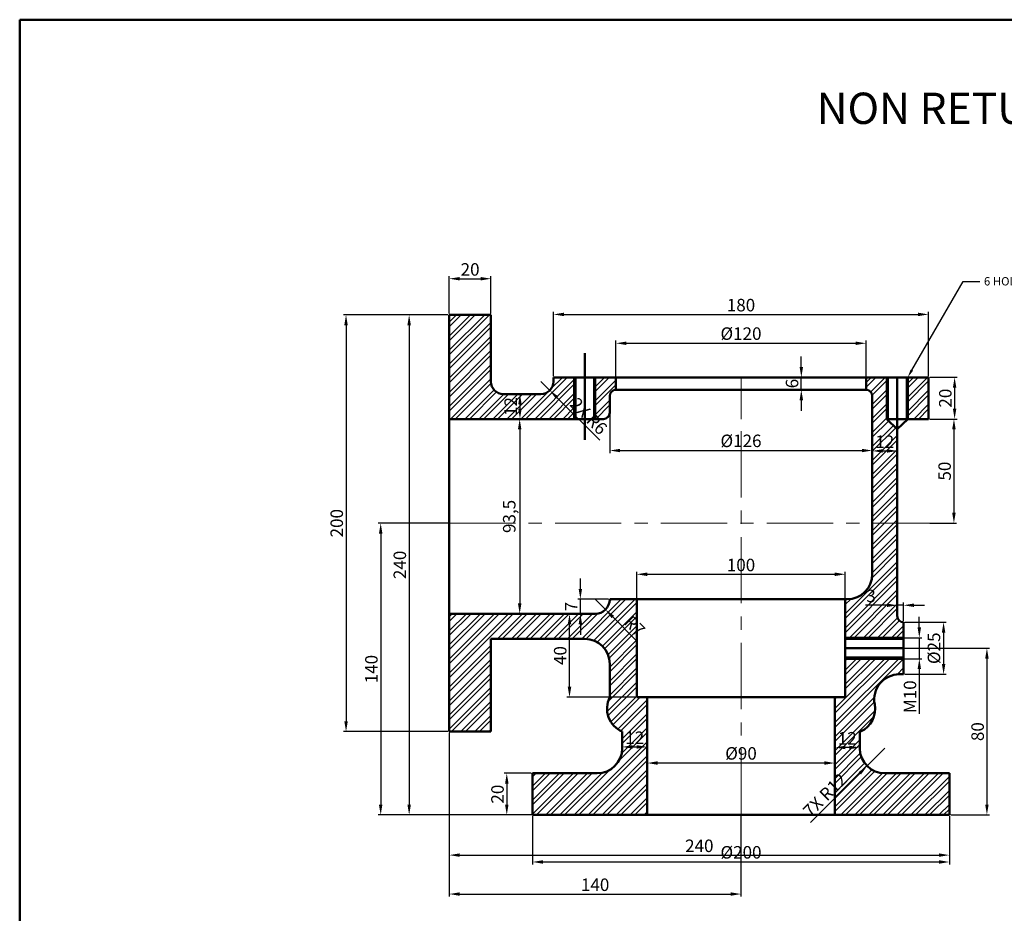
# Model space of a CAD drawing. Units: millimetres. Extents: x -907 to -46, y -312 to 510.
# Tile 2 of 3: x -907 to -434, y 81 to 510. Entities that reach past the tile are written whole.
import ezdxf
from ezdxf import colors
from ezdxf.entities.mleader import LeaderData, LeaderLine
from ezdxf.math import Vec2, Vec3

# ---------------------------------------------------------------- set-up
doc = ezdxf.new("R2010")
doc.units = ezdxf.units.MM
doc.linetypes.add('CENTER', pattern=[50.8, 31.75, -6.35, 6.35, -6.35])
for name, color, linetype, lineweight in [('M-CNTR', 1, 'CENTER', 18), ('M-DIMS', 2, 'Continuous', 25), ('M-HATC', 8, 'Continuous', 18), ('M-OUTL', 7, 'Continuous', 50), ('M-TEXT', 3, 'Continuous', 25), ('M-TTLB', 7, 'Continuous', 50)]:
    doc.layers.add(name, color=color, linetype=linetype, lineweight=lineweight)
doc.styles.get("Standard").update_dxf_attribs({"font": 'arial.ttf'})
doc.dimstyles.new('ISO-25', dxfattribs={"dimtxt": 6, "dimasz": 5, "dimexe": 1.25, "dimexo": 0.625, "dimtad": 1, "dimtxsty": 'Standard', "dimcen": 2.5, "dimadec": 0, "dimazin": 0, "dimtfac": 1, "dimtmove": 0, "dimatfit": 3, "dimfxl": 1, "dimarcsym": 0})

# ---------------------------------------------------------------- blocks, each defined once
blk = doc.blocks.new('*D1')
at = {"layer": 'Defpoints', "color": 0, "transparency": 16777216}
for p in [(-660.8, 128.33), (-460.8, 128.33), (-460.8, 105.78)]:
    blk.add_point(p, dxfattribs=at)
at = {"layer": 'M-DIMS', "color": 0, "lineweight": -2, "transparency": 16777216}
for p, q in [((-660.8, 127.7), (-660.8, 104.53)), ((-460.8, 127.7), (-460.8, 104.53)), ((-655.8, 105.78), (-465.8, 105.78))]:
    blk.add_line(p, q, dxfattribs=at)
at = {"layer": 'M-DIMS', "color": 0, "transparency": 16777216}
for points in [[(-655.8, 106.62), (-655.8, 104.95), (-660.8, 105.78)], [(-465.8, 106.62), (-465.8, 104.95), (-460.8, 105.78)]]:
    blk.add_solid(points, dxfattribs=at)
at = {"layer": 'M-DIMS', "color": 0, "transparency": 16777216, "insert": (-560.8, 109.64), "char_height": 6, "attachment_point": 5}
blk.add_mtext('%%C200', dxfattribs=at)
blk = doc.blocks.new('*D2')
at = {"layer": 'Defpoints', "color": 0, "transparency": 16777216}
for p in [(-700.8, 168.33), (-560.8, 128.33), (-560.8, 90.4)]:
    blk.add_point(p, dxfattribs=at)
at = {"layer": 'M-DIMS', "color": 0, "lineweight": -2, "transparency": 16777216}
for p, q in [((-700.8, 167.7), (-700.8, 89.15)), ((-560.8, 127.7), (-560.8, 89.15)), ((-695.8, 90.4), (-565.8, 90.4))]:
    blk.add_line(p, q, dxfattribs=at)
at = {"layer": 'M-DIMS', "color": 0, "transparency": 16777216}
for points in [[(-695.8, 91.23), (-695.8, 89.56), (-700.8, 90.4)], [(-565.8, 91.23), (-565.8, 89.56), (-560.8, 90.4)]]:
    blk.add_solid(points, dxfattribs=at)
at = {"layer": 'M-DIMS', "color": 0, "transparency": 16777216, "insert": (-630.8, 94.08), "char_height": 6, "attachment_point": 5}
blk.add_mtext('140', dxfattribs=at)
blk = doc.blocks.new('*D3')
at = {"layer": 'Defpoints', "color": 0, "transparency": 16777216}
for p in [(-605.8, 156.58), (-515.8, 156.58), (-605.8, 153.25)]:
    blk.add_point(p, dxfattribs=at)
at = {"layer": 'M-DIMS', "color": 0, "lineweight": -2, "transparency": 16777216}
for p, q in [((-605.8, 155.95), (-605.8, 152)), ((-515.8, 155.95), (-515.8, 152)), ((-520.8, 153.25), (-600.8, 153.25))]:
    blk.add_line(p, q, dxfattribs=at)
at = {"layer": 'M-DIMS', "color": 0, "transparency": 16777216}
for points in [[(-600.8, 154.09), (-600.8, 152.42), (-605.8, 153.25)], [(-520.8, 154.09), (-520.8, 152.42), (-515.8, 153.25)]]:
    blk.add_solid(points, dxfattribs=at)
at = {"layer": 'M-DIMS', "color": 0, "transparency": 16777216, "insert": (-560.8, 157.11), "char_height": 6, "attachment_point": 5}
blk.add_mtext('%%C90', dxfattribs=at)
blk = doc.blocks.new('*D4')
at = {"layer": 'Defpoints', "color": 0, "transparency": 16777216}
for p in [(-605.8, 160.99), (-617.8, 160.33), (-605.8, 160.33)]:
    blk.add_point(p, dxfattribs=at)
at = {"layer": 'M-DIMS', "color": 0, "lineweight": -2, "transparency": 16777216}
for p, q in [((-617.8, 160.95), (-617.8, 162.24)), ((-612.8, 160.99), (-610.8, 160.99)), ((-605.8, 160.95), (-605.8, 162.24))]:
    blk.add_line(p, q, dxfattribs=at)
at = {"layer": 'M-DIMS', "color": 0, "transparency": 16777216}
for points in [[(-612.8, 161.83), (-612.8, 160.16), (-617.8, 160.99)], [(-610.8, 161.83), (-610.8, 160.16), (-605.8, 160.99)]]:
    blk.add_solid(points, dxfattribs=at)
at = {"layer": 'M-DIMS', "color": 0, "transparency": 16777216, "insert": (-611.8, 164.63), "char_height": 6, "attachment_point": 5}
blk.add_mtext('12', dxfattribs=at)
blk = doc.blocks.new('*D5')
at = {"layer": 'Defpoints', "color": 0, "transparency": 16777216}
for p in [(-643.1, 224.83), (-630.8, 224.83), (-610.8, 184.83)]:
    blk.add_point(p, dxfattribs=at)
at = {"layer": 'M-DIMS', "color": 0, "lineweight": -2, "transparency": 16777216}
for p, q in [((-631.42, 224.83), (-644.35, 224.83)), ((-643.1, 189.83), (-643.1, 219.83)), ((-611.42, 184.83), (-644.35, 184.83))]:
    blk.add_line(p, q, dxfattribs=at)
at = {"layer": 'M-DIMS', "color": 0, "transparency": 16777216}
for points in [[(-643.93, 219.83), (-642.26, 219.83), (-643.1, 224.83)], [(-643.93, 189.83), (-642.26, 189.83), (-643.1, 184.83)]]:
    blk.add_solid(points, dxfattribs=at)
at = {"layer": 'M-DIMS', "color": 0, "transparency": 16777216, "insert": (-646.79, 204.83), "char_height": 6, "attachment_point": 5, "rotation": 90}
blk.add_mtext('40', dxfattribs=at)
blk = doc.blocks.new('*D6')
at = {"layer": 'Defpoints', "color": 0, "transparency": 16777216}
for p in [(-482.8, 208.33), (-460.8, 128.33), (-442.79, 128.33)]:
    blk.add_point(p, dxfattribs=at)
at = {"layer": 'M-DIMS', "color": 0, "lineweight": -2, "transparency": 16777216}
for p, q in [((-482.17, 208.33), (-441.54, 208.33)), ((-442.79, 203.33), (-442.79, 133.33)), ((-460.17, 128.33), (-441.54, 128.33))]:
    blk.add_line(p, q, dxfattribs=at)
at = {"layer": 'M-DIMS', "color": 0, "transparency": 16777216}
for points in [[(-443.62, 203.33), (-441.96, 203.33), (-442.79, 208.33)], [(-443.62, 133.33), (-441.96, 133.33), (-442.79, 128.33)]]:
    blk.add_solid(points, dxfattribs=at)
at = {"layer": 'M-DIMS', "color": 0, "transparency": 16777216, "insert": (-446.48, 168.33), "char_height": 6, "attachment_point": 5, "rotation": 90}
blk.add_mtext('80', dxfattribs=at)
blk = doc.blocks.new('*D7')
at = {"layer": 'Defpoints', "color": 0, "transparency": 16777216}
for p in [(-515.8, 164.33), (-515.8, 160.72), (-503.8, 164.33)]:
    blk.add_point(p, dxfattribs=at)
at = {"layer": 'M-DIMS', "color": 0, "lineweight": -2, "transparency": 16777216}
for p, q in [((-515.8, 163.7), (-515.8, 159.47)), ((-508.8, 160.72), (-510.8, 160.72)), ((-503.8, 163.7), (-503.8, 159.47))]:
    blk.add_line(p, q, dxfattribs=at)
at = {"layer": 'M-DIMS', "color": 0, "transparency": 16777216}
for points in [[(-510.8, 161.55), (-510.8, 159.89), (-515.8, 160.72)], [(-508.8, 161.55), (-508.8, 159.89), (-503.8, 160.72)]]:
    blk.add_solid(points, dxfattribs=at)
at = {"layer": 'M-DIMS', "color": 0, "transparency": 16777216, "insert": (-509.8, 164.36), "char_height": 6, "attachment_point": 5}
blk.add_mtext('12', dxfattribs=at)
blk = doc.blocks.new('*D8')
at = {"layer": 'Defpoints', "color": 0, "transparency": 16777216}
for p in [(-482.8, 213.33), (-482.8, 203.33), (-475.23, 203.33)]:
    blk.add_point(p, dxfattribs=at)
at = {"layer": 'M-DIMS', "color": 0, "lineweight": -2, "transparency": 16777216}
for p, q in [((-475.23, 218.33), (-475.23, 223.33)), ((-482.17, 213.33), (-473.98, 213.33)), ((-475.23, 213.33), (-475.23, 203.33)), ((-482.17, 203.33), (-473.98, 203.33)), ((-475.23, 198.33), (-475.23, 176.79))]:
    blk.add_line(p, q, dxfattribs=at)
at = {"layer": 'M-DIMS', "color": 0, "transparency": 16777216}
for points in [[(-476.06, 218.33), (-474.4, 218.33), (-475.23, 213.33)], [(-476.06, 198.33), (-474.4, 198.33), (-475.23, 203.33)]]:
    blk.add_solid(points, dxfattribs=at)
at = {"layer": 'M-DIMS', "color": 0, "transparency": 16777216, "insert": (-478.92, 185.06), "char_height": 6, "attachment_point": 5, "rotation": 90}
blk.add_mtext('M10', dxfattribs=at)
blk = doc.blocks.new('*D9')
at = {"layer": 'Defpoints', "color": 0, "transparency": 16777216}
for p in [(-482.8, 220.83), (-482.8, 195.83), (-463.58, 195.83)]:
    blk.add_point(p, dxfattribs=at)
at = {"layer": 'M-DIMS', "color": 0, "lineweight": -2, "transparency": 16777216}
for p, q in [((-482.17, 220.83), (-462.33, 220.83)), ((-463.58, 215.83), (-463.58, 200.83)), ((-482.17, 195.83), (-462.33, 195.83))]:
    blk.add_line(p, q, dxfattribs=at)
at = {"layer": 'M-DIMS', "color": 0, "transparency": 16777216}
for points in [[(-464.41, 215.83), (-462.74, 215.83), (-463.58, 220.83)], [(-464.41, 200.83), (-462.74, 200.83), (-463.58, 195.83)]]:
    blk.add_solid(points, dxfattribs=at)
at = {"layer": 'M-DIMS', "color": 0, "transparency": 16777216, "insert": (-467.43, 208.33), "char_height": 6, "attachment_point": 5, "rotation": 90}
blk.add_mtext('%%C25', dxfattribs=at)
blk = doc.blocks.new('*D10')
at = {"layer": 'Defpoints', "color": 0, "transparency": 16777216}
for p in [(-510.8, 243.83), (-610.8, 231.83), (-510.8, 231.83)]:
    blk.add_point(p, dxfattribs=at)
at = {"layer": 'M-DIMS', "color": 0, "lineweight": -2, "transparency": 16777216}
for p, q in [((-610.8, 232.45), (-610.8, 245.08)), ((-605.8, 243.83), (-515.8, 243.83)), ((-510.8, 232.45), (-510.8, 245.08))]:
    blk.add_line(p, q, dxfattribs=at)
at = {"layer": 'M-DIMS', "color": 0, "transparency": 16777216}
for points in [[(-605.8, 244.66), (-605.8, 242.99), (-610.8, 243.83)], [(-515.8, 244.66), (-515.8, 242.99), (-510.8, 243.83)]]:
    blk.add_solid(points, dxfattribs=at)
at = {"layer": 'M-DIMS', "color": 0, "transparency": 16777216, "insert": (-560.8, 247.51), "char_height": 6, "attachment_point": 5}
blk.add_mtext('100', dxfattribs=at)
blk = doc.blocks.new('*D11')
at = {"layer": 'Defpoints', "color": 0, "transparency": 16777216}
for p in [(-637.89, 231.83), (-623.8, 231.83), (-630.8, 224.83)]:
    blk.add_point(p, dxfattribs=at)
at = {"layer": 'M-DIMS', "color": 0, "lineweight": -2, "transparency": 16777216}
for p, q in [((-637.89, 236.83), (-637.89, 241.83)), ((-624.42, 231.83), (-639.14, 231.83)), ((-637.89, 224.83), (-637.89, 231.83)), ((-631.42, 224.83), (-639.14, 224.83)), ((-637.89, 219.83), (-637.89, 214.83))]:
    blk.add_line(p, q, dxfattribs=at)
at = {"layer": 'M-DIMS', "color": 0, "transparency": 16777216}
for points in [[(-638.72, 236.83), (-637.05, 236.83), (-637.89, 231.83)], [(-638.72, 219.83), (-637.05, 219.83), (-637.89, 224.83)]]:
    blk.add_solid(points, dxfattribs=at)
at = {"layer": 'M-DIMS', "color": 0, "transparency": 16777216, "insert": (-641.51, 228.33), "char_height": 6, "attachment_point": 5, "rotation": 90}
blk.add_mtext('7', dxfattribs=at)
blk = doc.blocks.new('*D12')
at = {"layer": 'Defpoints', "color": 0, "transparency": 16777216}
for p in [(-700.8, 268.33), (-733.7, 128.33), (-660.8, 128.33)]:
    blk.add_point(p, dxfattribs=at)
at = {"layer": 'M-DIMS', "color": 0, "lineweight": -2, "transparency": 16777216}
for p, q in [((-701.42, 268.33), (-734.95, 268.33)), ((-733.7, 263.33), (-733.7, 133.33)), ((-661.42, 128.33), (-734.95, 128.33))]:
    blk.add_line(p, q, dxfattribs=at)
at = {"layer": 'M-DIMS', "color": 0, "transparency": 16777216}
for points in [[(-734.54, 263.33), (-732.87, 263.33), (-733.7, 268.33)], [(-734.54, 133.33), (-732.87, 133.33), (-733.7, 128.33)]]:
    blk.add_solid(points, dxfattribs=at)
at = {"layer": 'M-DIMS', "color": 0, "transparency": 16777216, "insert": (-737.39, 198.33), "char_height": 6, "attachment_point": 5, "rotation": 90}
blk.add_mtext('140', dxfattribs=at)
blk = doc.blocks.new('*D13')
at = {"layer": 'Defpoints', "color": 0, "transparency": 16777216}
for p in [(-700.8, 368.33), (-750.33, 168.33), (-700.8, 168.33)]:
    blk.add_point(p, dxfattribs=at)
at = {"layer": 'M-DIMS', "color": 0, "lineweight": -2, "transparency": 16777216}
for p, q in [((-701.42, 368.33), (-751.58, 368.33)), ((-750.33, 363.33), (-750.33, 173.33)), ((-701.42, 168.33), (-751.58, 168.33))]:
    blk.add_line(p, q, dxfattribs=at)
at = {"layer": 'M-DIMS', "color": 0, "transparency": 16777216}
for points in [[(-751.16, 363.33), (-749.5, 363.33), (-750.33, 368.33)], [(-751.16, 173.33), (-749.5, 173.33), (-750.33, 168.33)]]:
    blk.add_solid(points, dxfattribs=at)
at = {"layer": 'M-DIMS', "color": 0, "transparency": 16777216, "insert": (-754.02, 268.33), "char_height": 6, "attachment_point": 5, "rotation": 90}
blk.add_mtext('200', dxfattribs=at)
blk = doc.blocks.new('*D14')
at = {"layer": 'Defpoints', "color": 0, "transparency": 16777216}
for p in [(-665.8, 330.33), (-666.88, 318.33), (-665.8, 318.33)]:
    blk.add_point(p, dxfattribs=at)
at = {"layer": 'M-DIMS', "color": 0, "lineweight": -2, "transparency": 16777216}
for p, q in [((-666.42, 330.33), (-668.13, 330.33)), ((-666.88, 325.33), (-666.88, 323.33)), ((-666.42, 318.33), (-668.13, 318.33))]:
    blk.add_line(p, q, dxfattribs=at)
at = {"layer": 'M-DIMS', "color": 0, "transparency": 16777216}
for points in [[(-667.72, 325.33), (-666.05, 325.33), (-666.88, 330.33)], [(-667.72, 323.33), (-666.05, 323.33), (-666.88, 318.33)]]:
    blk.add_solid(points, dxfattribs=at)
at = {"layer": 'M-DIMS', "color": 0, "transparency": 16777216, "insert": (-670.52, 324.33), "char_height": 6, "attachment_point": 5, "rotation": 90}
blk.add_mtext('12', dxfattribs=at)
blk = doc.blocks.new('*D15')
at = {"layer": 'Defpoints', "color": 0, "transparency": 16777216}
for p in [(-680.8, 385.65), (-700.8, 368.33), (-680.8, 368.33)]:
    blk.add_point(p, dxfattribs=at)
at = {"layer": 'M-DIMS', "color": 0, "lineweight": -2, "transparency": 16777216}
for p, q in [((-700.8, 368.95), (-700.8, 386.9)), ((-695.8, 385.65), (-685.8, 385.65)), ((-680.8, 368.95), (-680.8, 386.9))]:
    blk.add_line(p, q, dxfattribs=at)
at = {"layer": 'M-DIMS', "color": 0, "transparency": 16777216}
for points in [[(-695.8, 386.48), (-695.8, 384.81), (-700.8, 385.65)], [(-685.8, 386.48), (-685.8, 384.81), (-680.8, 385.65)]]:
    blk.add_solid(points, dxfattribs=at)
at = {"layer": 'M-DIMS', "color": 0, "transparency": 16777216, "insert": (-690.8, 389.33), "char_height": 6, "attachment_point": 5}
blk.add_mtext('20', dxfattribs=at)
blk = doc.blocks.new('*D16')
at = {"layer": 'Defpoints', "color": 0, "transparency": 16777216}
for p in [(-470.8, 368.52), (-650.8, 338.33), (-470.8, 338.33)]:
    blk.add_point(p, dxfattribs=at)
at = {"layer": 'M-DIMS', "color": 0, "lineweight": -2, "transparency": 16777216}
for p, q in [((-650.8, 338.95), (-650.8, 369.77)), ((-470.8, 338.95), (-470.8, 369.77)), ((-645.8, 368.52), (-475.8, 368.52))]:
    blk.add_line(p, q, dxfattribs=at)
at = {"layer": 'M-DIMS', "color": 0, "transparency": 16777216}
for points in [[(-645.8, 369.35), (-645.8, 367.68), (-650.8, 368.52)], [(-475.8, 369.35), (-475.8, 367.68), (-470.8, 368.52)]]:
    blk.add_solid(points, dxfattribs=at)
at = {"layer": 'M-DIMS', "color": 0, "transparency": 16777216, "insert": (-560.8, 372.2), "char_height": 6, "attachment_point": 5}
blk.add_mtext('180', dxfattribs=at)
blk = doc.blocks.new('*D17')
at = {"layer": 'Defpoints', "color": 0, "transparency": 16777216}
for p in [(-623.8, 321.33), (-497.8, 321.33), (-497.8, 303.21)]:
    blk.add_point(p, dxfattribs=at)
at = {"layer": 'M-DIMS', "color": 0, "lineweight": -2, "transparency": 16777216}
for p, q in [((-623.8, 320.7), (-623.8, 301.96)), ((-497.8, 320.7), (-497.8, 301.96)), ((-618.8, 303.21), (-502.8, 303.21))]:
    blk.add_line(p, q, dxfattribs=at)
at = {"layer": 'M-DIMS', "color": 0, "transparency": 16777216}
for points in [[(-618.8, 304.04), (-618.8, 302.38), (-623.8, 303.21)], [(-502.8, 304.04), (-502.8, 302.38), (-497.8, 303.21)]]:
    blk.add_solid(points, dxfattribs=at)
at = {"layer": 'M-DIMS', "color": 0, "transparency": 16777216, "insert": (-560.8, 307.07), "char_height": 6, "attachment_point": 5}
blk.add_mtext('%%C126', dxfattribs=at)
blk = doc.blocks.new('*D18')
at = {"layer": 'Defpoints', "color": 0, "transparency": 16777216}
for p in [(-470.8, 338.33), (-470.8, 318.33), (-458.29, 318.33)]:
    blk.add_point(p, dxfattribs=at)
at = {"layer": 'M-DIMS', "color": 0, "lineweight": -2, "transparency": 16777216}
for p, q in [((-470.17, 338.33), (-457.04, 338.33)), ((-458.29, 333.33), (-458.29, 323.33)), ((-470.17, 318.33), (-457.04, 318.33))]:
    blk.add_line(p, q, dxfattribs=at)
at = {"layer": 'M-DIMS', "color": 0, "transparency": 16777216}
for points in [[(-459.12, 333.33), (-457.46, 333.33), (-458.29, 338.33)], [(-459.12, 323.33), (-457.46, 323.33), (-458.29, 318.33)]]:
    blk.add_solid(points, dxfattribs=at)
at = {"layer": 'M-DIMS', "color": 0, "transparency": 16777216, "insert": (-461.98, 328.33), "char_height": 6, "attachment_point": 5, "rotation": 90}
blk.add_mtext('20', dxfattribs=at)
blk = doc.blocks.new('*D19')
at = {"layer": 'Defpoints', "color": 0, "transparency": 16777216}
for p in [(-500.8, 354.67), (-620.8, 332.33), (-500.8, 332.33)]:
    blk.add_point(p, dxfattribs=at)
at = {"layer": 'M-DIMS', "color": 0, "lineweight": -2, "transparency": 16777216}
for p, q in [((-620.8, 332.95), (-620.8, 355.92)), ((-615.8, 354.67), (-505.8, 354.67)), ((-500.8, 332.95), (-500.8, 355.92))]:
    blk.add_line(p, q, dxfattribs=at)
at = {"layer": 'M-DIMS', "color": 0, "transparency": 16777216}
for points in [[(-615.8, 355.5), (-615.8, 353.84), (-620.8, 354.67)], [(-505.8, 355.5), (-505.8, 353.84), (-500.8, 354.67)]]:
    blk.add_solid(points, dxfattribs=at)
at = {"layer": 'M-DIMS', "color": 0, "transparency": 16777216, "insert": (-560.8, 358.53), "char_height": 6, "attachment_point": 5}
blk.add_mtext('%%C120', dxfattribs=at)
blk = doc.blocks.new('*D20')
at = {"layer": 'Defpoints', "color": 0, "transparency": 16777216}
for p in [(-539.22, 338.33), (-531.85, 338.33), (-539.22, 332.33)]:
    blk.add_point(p, dxfattribs=at)
at = {"layer": 'M-DIMS', "color": 0, "lineweight": -2, "transparency": 16777216}
for p, q in [((-531.85, 343.33), (-531.85, 348.33)), ((-538.6, 338.33), (-530.6, 338.33)), ((-531.85, 332.33), (-531.85, 338.33)), ((-538.6, 332.33), (-530.6, 332.33)), ((-531.85, 327.33), (-531.85, 322.33))]:
    blk.add_line(p, q, dxfattribs=at)
at = {"layer": 'M-DIMS', "color": 0, "transparency": 16777216}
for points in [[(-532.68, 343.33), (-531.01, 343.33), (-531.85, 338.33)], [(-532.68, 327.33), (-531.01, 327.33), (-531.85, 332.33)]]:
    blk.add_solid(points, dxfattribs=at)
at = {"layer": 'M-DIMS', "color": 0, "transparency": 16777216, "insert": (-535.53, 335.33), "char_height": 6, "attachment_point": 5, "rotation": 90}
blk.add_mtext('6', dxfattribs=at)
blk = doc.blocks.new('*D21')
at = {"layer": 'Defpoints', "color": 0, "transparency": 16777216}
for p in [(-497.8, 306.37), (-485.8, 306.37), (-485.8, 303)]:
    blk.add_point(p, dxfattribs=at)
at = {"layer": 'M-DIMS', "color": 0, "lineweight": -2, "transparency": 16777216}
for p, q in [((-497.8, 305.74), (-497.8, 301.75)), ((-492.8, 303), (-490.8, 303)), ((-485.8, 305.74), (-485.8, 301.75))]:
    blk.add_line(p, q, dxfattribs=at)
at = {"layer": 'M-DIMS', "color": 0, "transparency": 16777216}
for points in [[(-492.8, 303.84), (-492.8, 302.17), (-497.8, 303)], [(-490.8, 303.84), (-490.8, 302.17), (-485.8, 303)]]:
    blk.add_solid(points, dxfattribs=at)
at = {"layer": 'M-DIMS', "color": 0, "transparency": 16777216, "insert": (-491.8, 306.64), "char_height": 6, "attachment_point": 5}
blk.add_mtext('12', dxfattribs=at)
blk = doc.blocks.new('*D22')
at = {"layer": 'Defpoints', "color": 0, "transparency": 16777216}
for p in [(-485.8, 228.96), (-485.8, 223.83), (-482.8, 220.83)]:
    blk.add_point(p, dxfattribs=at)
at = {"layer": 'M-DIMS', "color": 0, "lineweight": -2, "transparency": 16777216}
for p, q in [((-490.8, 228.96), (-500.98, 228.96)), ((-485.8, 224.45), (-485.8, 230.21)), ((-482.8, 228.96), (-485.8, 228.96)), ((-482.8, 221.45), (-482.8, 230.21)), ((-477.8, 228.96), (-472.8, 228.96))]:
    blk.add_line(p, q, dxfattribs=at)
at = {"layer": 'M-DIMS', "color": 0, "transparency": 16777216}
for points in [[(-490.8, 229.79), (-490.8, 228.12), (-485.8, 228.96)], [(-477.8, 229.79), (-477.8, 228.12), (-482.8, 228.96)]]:
    blk.add_solid(points, dxfattribs=at)
at = {"layer": 'M-DIMS', "color": 0, "transparency": 16777216, "insert": (-498.39, 232.65), "char_height": 6, "attachment_point": 5}
blk.add_mtext('3', dxfattribs=at)
blk = doc.blocks.new('*D23')
at = {"layer": 'Defpoints', "color": 0, "transparency": 16777216}
for p in [(-675.8, 318.33), (-675.8, 224.83), (-667, 224.83)]:
    blk.add_point(p, dxfattribs=at)
at = {"layer": 'M-DIMS', "color": 0, "lineweight": -2, "transparency": 16777216}
for p, q in [((-675.17, 318.33), (-665.75, 318.33)), ((-667, 313.33), (-667, 229.83)), ((-675.17, 224.83), (-665.75, 224.83))]:
    blk.add_line(p, q, dxfattribs=at)
at = {"layer": 'M-DIMS', "color": 0, "transparency": 16777216}
for points in [[(-667.84, 313.33), (-666.17, 313.33), (-667, 318.33)], [(-667.84, 229.83), (-666.17, 229.83), (-667, 224.83)]]:
    blk.add_solid(points, dxfattribs=at)
at = {"layer": 'M-DIMS', "color": 0, "transparency": 16777216, "insert": (-671.23, 271.58), "char_height": 6, "attachment_point": 5, "rotation": 90}
blk.add_mtext('93,5', dxfattribs=at)
blk = doc.blocks.new('*D44')
at = {"layer": 'Defpoints', "color": 0, "transparency": 16777216}
for p in [(-660.8, 148.33), (-673.19, 128.33), (-660.8, 128.33)]:
    blk.add_point(p, dxfattribs=at)
at = {"layer": 'M-DIMS', "color": 0, "lineweight": -2, "transparency": 16777216}
for p, q in [((-661.42, 148.33), (-674.44, 148.33)), ((-673.19, 143.33), (-673.19, 133.33)), ((-661.42, 128.33), (-674.44, 128.33))]:
    blk.add_line(p, q, dxfattribs=at)
at = {"layer": 'M-DIMS', "color": 0, "transparency": 16777216}
for points in [[(-674.02, 143.33), (-672.35, 143.33), (-673.19, 148.33)], [(-674.02, 133.33), (-672.35, 133.33), (-673.19, 128.33)]]:
    blk.add_solid(points, dxfattribs=at)
at = {"layer": 'M-DIMS', "color": 0, "transparency": 16777216, "insert": (-676.87, 138.33), "char_height": 6, "attachment_point": 5, "rotation": 90}
blk.add_mtext('20', dxfattribs=at)
blk = doc.blocks.new('*D45')
at = {"layer": 'Defpoints', "color": 0, "transparency": 16777216}
for p in [(-470.8, 318.33), (-470.8, 268.33), (-458.62, 268.33)]:
    blk.add_point(p, dxfattribs=at)
at = {"layer": 'M-DIMS', "color": 0, "lineweight": -2, "transparency": 16777216}
for p, q in [((-470.17, 318.33), (-457.37, 318.33)), ((-458.62, 313.33), (-458.62, 273.33)), ((-470.17, 268.33), (-457.37, 268.33))]:
    blk.add_line(p, q, dxfattribs=at)
at = {"layer": 'M-DIMS', "color": 0, "transparency": 16777216}
for points in [[(-459.46, 313.33), (-457.79, 313.33), (-458.62, 318.33)], [(-459.46, 273.33), (-457.79, 273.33), (-458.62, 268.33)]]:
    blk.add_solid(points, dxfattribs=at)
at = {"layer": 'M-DIMS', "color": 0, "transparency": 16777216, "insert": (-462.31, 293.33), "char_height": 6, "attachment_point": 5, "rotation": 90}
blk.add_mtext('50', dxfattribs=at)
blk = doc.blocks.new('*D55')
at = {"layer": 'Defpoints', "color": 0, "transparency": 16777216}
for p in [(-700.8, 368.33), (-720.05, 128.33), (-460.8, 128.33)]:
    blk.add_point(p, dxfattribs=at)
at = {"layer": 'M-DIMS', "color": 0, "lineweight": -2, "transparency": 16777216}
for p, q in [((-701.42, 368.33), (-721.3, 368.33)), ((-720.05, 363.33), (-720.05, 133.33)), ((-461.42, 128.33), (-721.3, 128.33))]:
    blk.add_line(p, q, dxfattribs=at)
at = {"layer": 'M-DIMS', "color": 0, "transparency": 16777216}
for points in [[(-720.88, 363.33), (-719.21, 363.33), (-720.05, 368.33)], [(-720.88, 133.33), (-719.21, 133.33), (-720.05, 128.33)]]:
    blk.add_solid(points, dxfattribs=at)
at = {"layer": 'M-DIMS', "color": 0, "transparency": 16777216, "insert": (-723.74, 248.33), "char_height": 6, "attachment_point": 5, "rotation": 90}
blk.add_mtext('240', dxfattribs=at)
blk = doc.blocks.new('*D56')
at = {"layer": 'Defpoints', "color": 0, "transparency": 16777216}
for p in [(-700.8, 168.33), (-460.8, 128.33), (-460.8, 109.08)]:
    blk.add_point(p, dxfattribs=at)
at = {"layer": 'M-DIMS', "color": 0, "lineweight": -2, "transparency": 16777216}
for p, q in [((-700.8, 167.7), (-700.8, 107.83)), ((-460.8, 127.7), (-460.8, 107.83)), ((-695.8, 109.08), (-465.8, 109.08))]:
    blk.add_line(p, q, dxfattribs=at)
at = {"layer": 'M-DIMS', "color": 0, "transparency": 16777216}
for points in [[(-695.8, 109.91), (-695.8, 108.24), (-700.8, 109.08)], [(-465.8, 109.91), (-465.8, 108.24), (-460.8, 109.08)]]:
    blk.add_solid(points, dxfattribs=at)
at = {"layer": 'M-DIMS', "color": 0, "transparency": 16777216, "insert": (-580.8, 112.76), "char_height": 6, "attachment_point": 5}
blk.add_mtext('240', dxfattribs=at)
blk = doc.blocks.new('*D61')
at = {"layer": 'Defpoints', "color": 0, "transparency": 16777216}
for p in [(-491.8, 160.33), (-500.28, 151.84)]:
    blk.add_point(p, dxfattribs=at)
at = {"layer": 'M-DIMS', "color": 0, "lineweight": -2, "transparency": 16777216}
for p, q in [((-491.8, 160.33), (-500.28, 151.84)), ((-527.41, 124.71), (-503.82, 148.3))]:
    blk.add_line(p, q, dxfattribs=at)
at = {"layer": 'M-DIMS', "color": 0, "transparency": 16777216}
blk.add_solid([(-504.41, 148.89), (-503.23, 147.72), (-500.28, 151.84)], dxfattribs=at)
at = {"layer": 'M-DIMS', "color": 0, "transparency": 16777216, "insert": (-519.96, 137.31), "char_height": 6, "attachment_point": 5, "rotation": 44.9999}
blk.add_mtext('7X R12', dxfattribs=at)
blk = doc.blocks.new('*D62')
at = {"layer": 'Defpoints', "color": 0, "transparency": 16777216}
for p in [(-630.8, 231.83), (-625.85, 226.88)]:
    blk.add_point(p, dxfattribs=at)
at = {"layer": 'M-DIMS', "color": 0, "lineweight": -2, "transparency": 16777216}
for p, q in [((-630.8, 231.83), (-625.85, 226.88)), ((-611.05, 212.08), (-622.31, 223.34))]:
    blk.add_line(p, q, dxfattribs=at)
at = {"layer": 'M-DIMS', "color": 0, "transparency": 16777216}
blk.add_solid([(-621.72, 223.93), (-622.9, 222.75), (-625.85, 226.88)], dxfattribs=at)
at = {"layer": 'M-DIMS', "color": 0, "transparency": 16777216, "insert": (-612.35, 218.51), "char_height": 6, "attachment_point": 5, "rotation": 315.0025}
blk.add_mtext('R7', dxfattribs=at)
blk = doc.blocks.new('*D63')
at = {"layer": 'Defpoints', "color": 0, "transparency": 16777216}
for p in [(-656.8, 336.33), (-652.55, 332.08)]:
    blk.add_point(p, dxfattribs=at)
at = {"layer": 'M-DIMS', "color": 0, "lineweight": -2, "transparency": 16777216}
for p, q in [((-656.8, 336.33), (-652.55, 332.08)), ((-628.57, 308.1), (-649.02, 328.55))]:
    blk.add_line(p, q, dxfattribs=at)
at = {"layer": 'M-DIMS', "color": 0, "transparency": 16777216}
blk.add_solid([(-648.43, 329.14), (-649.61, 327.96), (-652.55, 332.08)], dxfattribs=at)
at = {"layer": 'M-DIMS', "color": 0, "transparency": 16777216, "insert": (-634.42, 319.17), "char_height": 6, "attachment_point": 5, "rotation": 315.0029}
blk.add_mtext('2X R6', dxfattribs=at)

msp = doc.modelspace()

# ---------------------------------------------------------------- hatches: boundary and pattern name
at = {"layer": 'M-HATC'}
h = msp.add_hatch(dxfattribs=at)
h.set_pattern_fill('ANSI32', color=256, scale=0.5)
h.set_pattern_definition([(45, (-795.1453, -59.568), (-3.367596, 3.367596), []), (45, (-792.9, -59.568), (-3.367596, 3.367596), [])])
h.paths.add_polyline_path([(-640.7977, 338.3253), (-650.7977, 338.3253), (-650.7977, 336.3253, -0.41421356), (-656.7977, 330.3253), (-674.7977, 330.3253, -0.41421356), (-680.7977, 336.3253), (-680.7977, 368.3253), (-700.7977, 368.3253), (-700.7977, 318.3253), (-650.7977, 318.3253), (-640.7977, 318.3253)])
h.paths.add_polyline_path([(-620.7977, 338.3253), (-630.7977, 338.3253), (-630.7977, 318.3253), (-626.7977, 318.3253, 0.41421356), (-623.7977, 321.3253), (-623.7977, 329.3253, -0.41421356), (-620.7977, 332.3253)])
h.paths.add_polyline_path([(-490.7977, 338.3253), (-500.7977, 338.3253), (-500.7977, 332.3253, -0.41421356), (-497.7977, 329.3253), (-497.7977, 268.3253), (-485.7977, 268.3253), (-485.7977, 313.441), (-490.7977, 318.3253)])
h.paths.add_polyline_path([(-470.7977, 338.3253), (-480.7977, 338.3253), (-480.7977, 318.3253), (-470.7977, 318.3253)])
h.paths.add_polyline_path([(-605.7977, 184.8253), (-610.7977, 184.8253), (-610.7977, 231.8253), (-623.7977, 231.8253, -0.41421356), (-630.7977, 224.8253), (-700.7977, 224.8253), (-700.7977, 168.3253), (-680.7977, 168.3253), (-680.7977, 212.8253), (-635.7977, 212.8253, -0.41421356), (-623.7977, 200.8253), (-623.7977, 184.8253), (-623.7672, 184.8253, 0.43460042), (-617.7977, 168.3253), (-617.7977, 160.3253, -0.41421356), (-629.7977, 148.3253), (-660.7977, 148.3253), (-660.7977, 128.3253), (-605.7977, 128.3253)])
h.paths.add_polyline_path([(-460.7977, 148.3253), (-491.7977, 148.3253, -0.41421356), (-503.7977, 160.3253), (-503.7977, 168.3253), (-503.3904, 168.3253, 0.34589448), (-496.6331, 181.525, -0.47190523), (-484.8557, 195.8253), (-482.7977, 195.8253), (-482.7977, 203.3253), (-510.7977, 203.3253), (-510.7977, 184.8253), (-515.7977, 184.8253), (-515.7977, 128.3253), (-460.7977, 128.3253)])
h.paths.add_polyline_path([(-485.7977, 223.8253), (-485.7977, 268.3253), (-497.7977, 268.3253), (-497.7977, 243.8253, -0.41421356), (-509.7977, 231.8253), (-510.7977, 231.8253), (-510.7977, 213.3253), (-482.7977, 213.3253), (-482.7977, 220.8253, -0.41421356)])
h.paths.add_polyline_path([(-618.1947, 158.3417), (-605.8714, 158.3417), (-605.8714, 170.706), (-618.1947, 170.706)], flags=25)
h.paths.add_polyline_path([(-516.1947, 158.0678), (-503.8714, 158.0678), (-503.8714, 170.4321), (-516.1947, 170.4321)], flags=9)
h.paths.add_polyline_path([(-500.2037, 226.4105), (-492.5421, 226.4105), (-492.5421, 238.7748), (-500.2037, 238.7748)], flags=24)

# ---------------------------------------------------------------- linework, layer by layer
at = {"layer": 'M-CNTR'}
for p, q in [((-560.7977, 318.3253), (-560.7977, 338.3253)), ((-560.7977, 128.3253), (-560.7977, 318.3253)), ((-700.7977, 268.3253), (-460.7977, 268.3253))]:
    msp.add_line(p, q, dxfattribs=at)
at = {"layer": 'M-OUTL'}
for p, q in [((-700.7977, 168.3253), (-700.7977, 368.3253)), ((-700.7977, 368.3253), (-680.7977, 368.3253)), ((-680.7977, 368.3253), (-680.7977, 336.3253)), ((-635.7977, 349.9121), (-635.7977, 308.2882)), ((-650.7977, 336.3253), (-650.7977, 338.3253)), ((-650.7977, 338.3253), (-560.7977, 338.3253)), ((-640.7977, 338.3253), (-640.7977, 318.3253)), ((-640.2977, 338.3253), (-640.2977, 318.3253)), ((-635.7977, 338.3253), (-635.7977, 318.3253)), ((-635.7977, 338.3253), (-635.7977, 318.3253)), ((-635.7977, 338.3253), (-635.7977, 318.3253)), ((-631.2977, 338.3253), (-631.2977, 318.3253)), ((-630.7977, 338.3253), (-630.7977, 318.3253)), ((-620.7977, 332.3253), (-620.7977, 338.3253)), ((-560.7977, 338.3253), (-470.7977, 338.3253)), ((-500.7977, 332.3253), (-500.7977, 338.3253)), ((-490.7977, 318.3253), (-490.7977, 338.3253)), ((-490.2977, 317.8368), (-490.2977, 338.3253)), ((-485.7977, 318.3253), (-485.7977, 338.3253)), ((-481.2977, 317.8368), (-481.2977, 338.3253)), ((-480.7977, 318.3253), (-480.7977, 338.3253)), ((-470.7977, 318.3253), (-470.7977, 338.3253)), ((-620.7977, 332.3253), (-500.7977, 332.3253)), ((-674.7977, 330.3253), (-656.7977, 330.3253)), ((-623.7977, 321.3253), (-623.7977, 329.3253)), ((-497.7977, 243.8253), (-497.7977, 329.3253)), ((-700.7977, 318.3253), (-650.7977, 318.3253)), ((-650.7977, 318.3253), (-626.7977, 318.3253)), ((-490.7977, 318.3253), (-485.7977, 313.441)), ((-490.7977, 318.3253), (-470.7977, 318.3253)), ((-485.7977, 223.8253), (-485.7977, 318.3253)), ((-480.7977, 318.3253), (-485.7977, 313.441)), ((-623.7977, 231.8253), (-509.7977, 231.8253)), ((-623.7977, 231.8253), (-623.7977, 231.8253)), ((-610.7977, 184.8253), (-610.7977, 231.8253)), ((-510.7977, 184.8253), (-510.7977, 231.8253)), ((-700.7977, 224.8253), (-630.7977, 224.8253)), ((-482.7977, 220.8253), (-482.7977, 220.8253)), ((-482.7977, 195.8253), (-482.7977, 220.8253)), ((-680.7977, 212.8253), (-635.7977, 212.8253)), ((-680.7977, 212.8253), (-680.7977, 168.3253)), ((-510.7977, 213.3253), (-482.7977, 213.3253)), ((-510.7977, 212.8253), (-482.7977, 212.8253)), ((-510.7977, 208.3253), (-482.7977, 208.3253)), ((-510.7977, 208.3253), (-482.7977, 208.3253)), ((-510.7977, 203.8253), (-482.7977, 203.8253)), ((-510.7977, 203.3253), (-482.7977, 203.3253)), ((-623.7977, 184.7652), (-623.7977, 200.8253)), ((-484.8557, 195.8253), (-482.7977, 195.8253)), ((-623.7977, 184.8253), (-623.7672, 184.8253)), ((-610.7977, 184.8253), (-510.7977, 184.8253)), ((-605.7977, 128.3253), (-605.7977, 184.8253)), ((-515.7977, 128.3253), (-515.7977, 184.8253)), ((-700.7977, 168.3253), (-680.7977, 168.3253)), ((-617.7977, 160.3253), (-617.7977, 168.3253)), ((-503.7977, 160.3253), (-503.7977, 168.3253)), ((-503.7977, 168.3253), (-503.3904, 168.3253)), ((-660.7977, 148.3253), (-660.7977, 128.3253)), ((-629.7977, 148.3253), (-660.7977, 148.3253)), ((-460.7977, 148.3253), (-491.7977, 148.3253)), ((-460.7977, 128.3253), (-460.7977, 148.3253)), ((-660.7977, 128.3253), (-460.7977, 128.3253))]:
    msp.add_line(p, q, dxfattribs=at)
for centre, radius, start, end in [((-674.7977, 336.3253), 6, 180, 270), ((-656.7977, 336.3253), 6, 270, 0), ((-620.7977, 329.3253), 3, 90, 180), ((-500.7977, 329.3253), 3, 0, 90), ((-626.7977, 321.3253), 3, 270, 0), ((-509.7977, 243.8253), 12, 270, 0), ((-630.7977, 231.8253), 7, 270, 0), ((-482.7977, 223.8253), 3, 180, 270), ((-635.7977, 200.8253), 12, 0, 90), ((-484.8557, 183.8253), 12, 90, 191.051479), ((-613.0837, 179.3606), 12, 152.909955, 246.869099), ((-508.4106, 179.2247), 12, 294.730597, 11.051479), ((-629.7977, 160.3253), 12, 270, 0), ((-491.7977, 160.3253), 12, 180, 270)]:
    msp.add_arc(centre, radius, start, end, dxfattribs=at)
at = {"layer": 'M-TTLB'}
msp.add_lwpolyline([(-906.9397, 509.9283), (-45.5255, 509.9283), (-45.5255, -312.1438), (-906.9397, -312.1438)], close=True, dxfattribs=at)

# ---------------------------------------------------------------- texts
at = {"layer": 'M-TEXT', "insert": (-644.8993, 474.9186), "char_height": 15, "attachment_point": 1}
msp.add_mtext_dynamic_manual_height_columns('\\pxqc;NON RETURN VALVE', width=433.762066, gutter_width=12.5, heights=[0], dxfattribs=at)

# ---------------------------------------------------------------- dimensions: what is measured, and where the dimension line sits
at = {"layer": 'M-DIMS'}
for base, p1, p2, override, picture, middle in [((-680.7977, 385.6458), (-700.7977, 368.3253), (-680.7977, 368.3253), {"dimclrd": 0, "dimclre": 0, "dimclrt": 0}, '*D15', (-690.7977, 389.3342)), ((-470.7977, 368.5151), (-650.7977, 338.3253), (-470.7977, 338.3253), {"dimclrd": 0, "dimclre": 0, "dimclrt": 0}, '*D16', (-560.7977, 372.2035)), ((-485.7977, 303.0017), (-497.7977, 306.3654), (-485.7977, 306.3654), {"dimclrd": 0, "dimclre": 0, "dimclrt": 0}, '*D21', (-491.7977, 306.639)), ((-510.7977, 243.8253), (-610.7977, 231.8253), (-510.7977, 231.8253), {"dimclrd": 0, "dimclre": 0, "dimclrt": 0}, '*D10', (-560.7977, 247.5137)), ((-485.7977, 228.9553), (-482.7977, 220.8253), (-485.7977, 223.8253), {"dimclrd": 0, "dimclre": 0, "dimclrt": 0}, '*D22', (-498.3872, 232.6458)), ((-560.7977, 90.3956), (-700.7977, 168.3253), (-560.7977, 128.3253), {"dimclrd": 0, "dimclre": 0, "dimclrt": 0}, '*D2', (-630.7977, 94.084)), ((-460.7977, 109.0753), (-700.7977, 168.3253), (-460.7977, 128.3253), {"dimdec": 0, "dimlfac": 1, "dimrnd": 0, "dimzin": 0, "dimdsep": 46, "dimlunit": 2}, '*D56', (-580.7977, 112.7637)), ((-605.7977, 160.993), (-617.7977, 160.3253), (-605.7977, 160.3253), {"dimclrd": 0, "dimclre": 0, "dimclrt": 0}, '*D4', (-611.7977, 164.6303)), ((-515.7977, 160.7191), (-503.7977, 164.3253), (-515.7977, 164.3253), {"dimclrd": 0, "dimclre": 0, "dimclrt": 0}, '*D7', (-509.7977, 164.3564))]:
    dim = msp.add_linear_dim(base=base, p1=p1, p2=p2, dimstyle='ISO-25', override=override, dxfattribs=at)
    dim.commit()
    dim.dimension.update_dxf_attribs({"geometry": picture, "text_midpoint": middle})
for base, p1, p2, override, picture, middle in [((-750.3306, 168.3253), (-700.7977, 368.3253), (-700.7977, 168.3253), {"dimclrd": 0, "dimclre": 0, "dimclrt": 0}, '*D13', (-754.019, 268.3253)), ((-720.0477, 128.3253), (-700.7977, 368.3253), (-460.7977, 128.3253), {"dimdec": 0, "dimlfac": 1, "dimrnd": 0, "dimzin": 0, "dimdsep": 46, "dimlunit": 2}, '*D55', (-723.7361, 248.3253)), ((-531.8453, 338.3253), (-539.2219, 332.3253), (-539.2219, 338.3253), {"dimclrd": 0, "dimclre": 0, "dimclrt": 0}, '*D20', (-535.5338, 335.3253)), ((-458.2913, 318.3253), (-470.7977, 338.3253), (-470.7977, 318.3253), {"dimclrd": 0, "dimclre": 0, "dimclrt": 0}, '*D18', (-461.9797, 328.3253)), ((-666.8835, 318.3253), (-665.7977, 330.3253), (-665.7977, 318.3253), {"dimclrd": 0, "dimclre": 0, "dimclrt": 0}, '*D14', (-670.5207, 324.3253)), ((-667.0026, 224.8253), (-675.7977, 318.3253), (-675.7977, 224.8253), {"dimclrd": 0, "dimclre": 0, "dimclrt": 0}, '*D23', (-671.2333, 271.5753)), ((-458.6246, 268.3253), (-470.7977, 318.3253), (-470.7977, 268.3253), {"dimclrd": 0, "dimclre": 0, "dimclrt": 0}, '*D45', (-462.3131, 293.3253)), ((-733.7046, 128.3253), (-700.7977, 268.3253), (-660.7977, 128.3253), {"dimclrd": 0, "dimclre": 0, "dimclrt": 0}, '*D12', (-737.3931, 198.3253)), ((-637.8852, 231.8253), (-630.7977, 224.8253), (-623.7977, 231.8253), {"dimclrd": 0, "dimclre": 0, "dimclrt": 0}, '*D11', (-641.5102, 228.3253)), ((-643.0977, 224.8253), (-610.7977, 184.8253), (-630.7977, 224.8253), {"dimclrd": 0, "dimclre": 0, "dimclrt": 0}, '*D5', (-646.7862, 204.8253)), ((-442.7899, 128.3253), (-482.7977, 208.3253), (-460.7977, 128.3253), {"dimclrd": 0, "dimclre": 0, "dimclrt": 0}, '*D6', (-446.4783, 168.3253)), ((-673.1855, 128.3253), (-660.7977, 148.3253), (-660.7977, 128.3253), {"dimclrd": 0, "dimclre": 0, "dimclrt": 0}, '*D44', (-676.874, 138.3253))]:
    dim = msp.add_linear_dim(base=base, p1=p1, p2=p2, angle=90, dimstyle='ISO-25', override=override, dxfattribs=at)
    dim.commit()
    dim.dimension.update_dxf_attribs({"geometry": picture, "text_midpoint": middle})
for base, p1, p2, picture, middle in [((-500.7977, 354.6707), (-620.7977, 332.3253), (-500.7977, 332.3253), '*D19', (-560.7977, 358.527)), ((-497.7977, 303.211), (-623.7977, 321.3253), (-497.7977, 321.3253), '*D17', (-560.7977, 307.0672)), ((-605.7977, 153.2534), (-515.7977, 156.5753), (-605.7977, 156.5753), '*D3', (-560.7977, 157.1097)), ((-460.7977, 105.785), (-660.7977, 128.3253), (-460.7977, 128.3253), '*D1', (-560.7977, 109.6412))]:
    dim = msp.add_linear_dim(base=base, p1=p1, p2=p2, text='%%C<>', dimstyle='ISO-25', override={"dimclrd": 0, "dimclre": 0, "dimclrt": 0}, dxfattribs=at)
    dim.commit()
    dim.dimension.update_dxf_attribs({"geometry": picture, "text_midpoint": middle})
for center, mpoint, text, picture, middle in [((-656.7977, 336.3253), (-652.5548, 332.0828), '2X <>', '*D63', (-634.4195, 319.1653)), ((-491.7977, 160.3253), (-500.283, 151.84), '7X <>', '*D61', (-519.9573, 137.3125))]:
    dim = msp.add_radius_dim(center=center, mpoint=mpoint, text=text, dimstyle='ISO-25', override={"dimdec": 0, "dimlfac": 1, "dimrnd": 0, "dimzin": 0, "dimdsep": 46, "dimlunit": 2}, dxfattribs=at)
    dim.commit()
    dim.dimension.update_dxf_attribs({"geometry": picture, "text_midpoint": middle})
dim = msp.add_radius_dim(center=(-630.7977, 231.8253), mpoint=(-625.8477, 226.8757), dimstyle='ISO-25', override={"dimdec": 0, "dimlfac": 1, "dimrnd": 0, "dimzin": 0, "dimdsep": 46, "dimlunit": 2}, dxfattribs=at)
dim.commit()
dim.dimension.update_dxf_attribs({"geometry": '*D62', "text_midpoint": (-612.3504, 218.5058)})
for base, p1, p2, text, picture, middle in [((-475.2284, 203.3253), (-482.7977, 213.3253), (-482.7977, 203.3253), 'M<>', '*D8', (-478.9168, 185.0591)), ((-463.5769, 195.8253), (-482.7977, 220.8253), (-482.7977, 195.8253), '%%C<>', '*D9', (-467.4331, 208.3253))]:
    dim = msp.add_linear_dim(base=base, p1=p1, p2=p2, angle=90, text=text, dimstyle='ISO-25', override={"dimclrd": 0, "dimclre": 0, "dimclrt": 0}, dxfattribs=at)
    dim.commit()
    dim.dimension.update_dxf_attribs({"geometry": picture, "text_midpoint": middle})

# ---------------------------------------------------------------- leaders
ml = msp.add_multileader_mtext('Standard', dxfattribs=at)
ml.set_content('6 HOLES M.16 PCD 150', color=256)
ml.set_leader_properties()
ml.build(insert=Vec2(0, 0))
ctx = ml.context
ctx.base_point, ctx.plane_origin = Vec3(-446.2087, 384.3788), Vec3(-480.7977, 338.3253)
notes = []
notes.append((ctx, [(0, (1, 1, 0), (-454.2087, 384.3788), (1, 0), 8, [(0, [(-480.7977, 338.3253)], 0, [])])]))
ctx.mtext.insert, ctx.mtext.flow_direction = Vec3(-444.2087, 386.4129), 5
for ctx, leaders in notes:
    for number, flags, end, landing, length, lines in leaders:
        leader = LeaderData()
        leader.index, (leader.has_last_leader_line, leader.has_dogleg_vector, leader.attachment_direction) = number, flags
        leader.last_leader_point, leader.dogleg_vector, leader.dogleg_length = Vec3(end), Vec3(landing), length
        for number, points, colour, breaks in lines:
            line = LeaderLine()
            line.index, line.vertices, line.color, line.breaks = number, Vec3.list(points), colors.encode_raw_color(colour), breaks
            leader.lines.append(line)
        ctx.leaders.append(leader)

doc.saveas('drawing.dxf')
